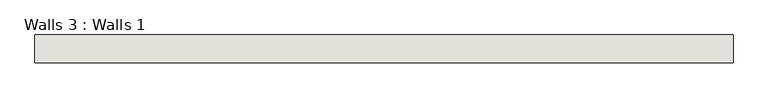
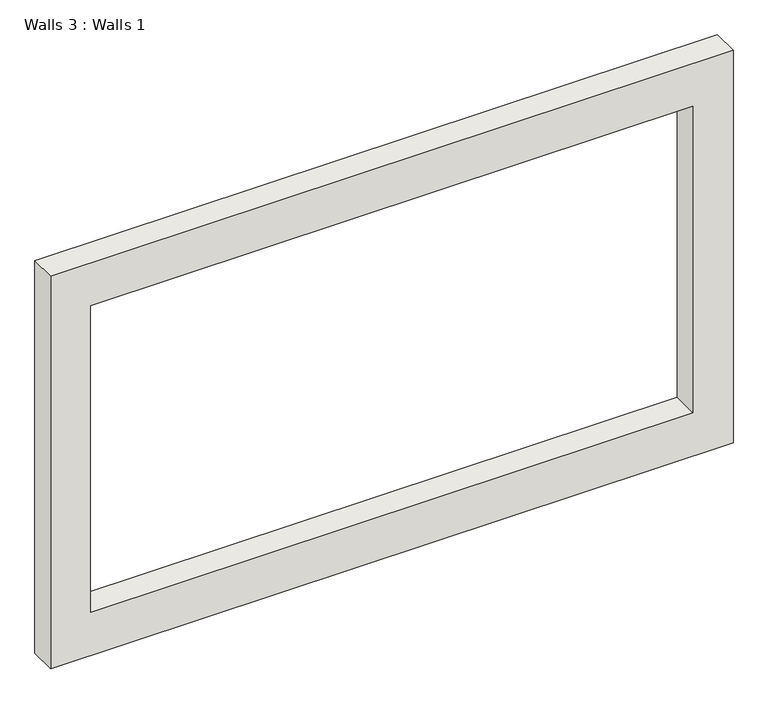
"""IFC4 building model written with IfcOpenShell, lengths in millimetres: wall geometry, Walls 3 : Walls 1."""

from ifc_helpers import new_model, si_unit, frame, origin, place, context, project, spatial, polyline, outline, extrude, source, transform, mapped, element, save


def walls_3_walls_1_a56c50be(model_context):
    return source(origin(), model_context, "Body", "SweptSolid", [
        extrude(outline(polyline([(17634.5693979, 1712.6958607), (17634.5693979, -878.1041393), (16059.7693979, -878.1041393), (16059.7693979, 1712.6958607), (17634.5693979, 1712.6958607)]), holes=[polyline([(17464.824337, 1560.0533085), (16233.9422066, 1560.0533085), (16233.9422066, -725.9466915), (17464.824337, -725.9466915), (17464.824337, 1560.0533085)])]), frame((0.0, -4092.2983041, 0.0), z_axis=(0.0, 1.0, 0.0), x_axis=(0.0, 0.0, 1.0)), (0.0, 0.0, 1.0), 103.0657287),
    ])


if __name__ == "__main__":
    model = new_model("IFC4")
    model_context = context("Model", 3, world=origin())
    ifc_project = project(units=[si_unit("LENGTHUNIT", "METRE", prefix="MILLI")], contexts=[model_context])
    site = spatial("IfcSite", under=ifc_project)
    building = spatial("IfcBuilding", under=site)
    placement = place(None, origin())
    walls_3_walls_1_shape = walls_3_walls_1_a56c50be(model_context)
    element("IfcWall", 1, ObjectType="Walls 3 : Walls 1", at=placement, inside=building, context=model_context, shape_type="MappedRepresentation", body=[
        mapped(walls_3_walls_1_shape, transform((0.0, 0.0, 0.0), x_axis=(1.0, 0.0, 0.0), y_axis=(0.0, 1.0, 0.0), z_axis=(0.0, 0.0, 1.0))),
    ])
    save(model, "model.ifc")

# Revit data of these elements
# Element 1 (IfcWall, "Walls 3 : Walls 1")
#   Materials on its faces: "Default Wall"
# Materials
#   "Default Wall": colour RGB 128 128 128, transparency 0
